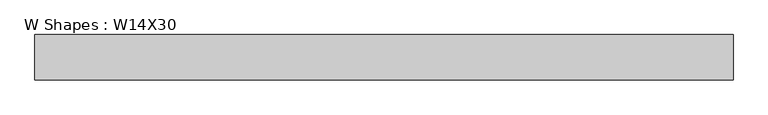
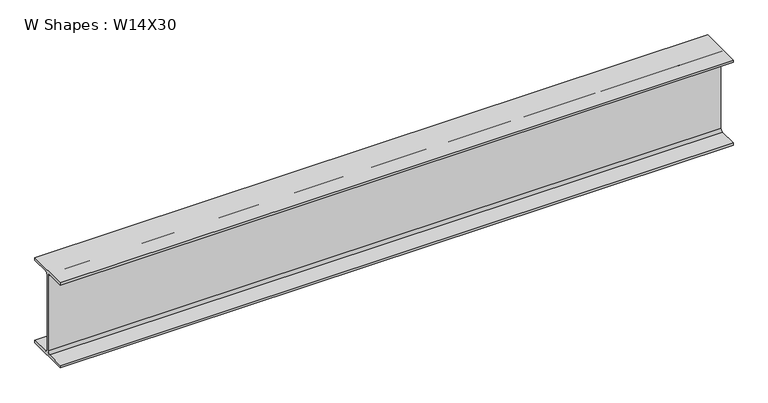
"""IFC4 building model written with IfcOpenShell, lengths in millimetres: beam geometry, W Shapes : W14X30."""

from ifc_helpers import new_model, si_unit, point, frame, frame_2d, origin, place, context, project, spatial, polyline, circle_curve, trimmed, segment, composite_curve, outline, extrude, source, transform, mapped, element, save


def w_shapes_w14x30_e8a2e8cf(model_context):
    return source(origin(), model_context, "Body", "SweptSolid", [
        extrude(outline(composite_curve([segment(polyline([(85.471, -165.481), (85.471, -175.26), (-85.471, -175.26), (-85.471, -165.481), (-13.589, -165.481)]), True, "CONTINUOUS"), segment(trimmed(circle_curve(frame_2d((-13.589, -155.321)), 10.16), [point((-13.589, -165.481))], [point((-3.429, -155.321))], True, "CARTESIAN"), True, "CONTINUOUS"), segment(polyline([(-3.429, -155.321), (-3.429, 155.321)]), True, "CONTINUOUS"), segment(trimmed(circle_curve(frame_2d((-13.589, 155.321)), 10.16), [point((-3.429, 155.321))], [point((-13.589, 165.481))], True, "CARTESIAN"), True, "CONTINUOUS"), segment(polyline([(-13.589, 165.481), (-85.471, 165.481), (-85.471, 175.26), (85.471, 175.26), (85.471, 165.481), (13.589, 165.481)]), True, "CONTINUOUS"), segment(trimmed(circle_curve(frame_2d((13.589, 155.321)), 10.16), [point((13.589, 165.481))], [point((3.429, 155.321))], True, "CARTESIAN"), True, "CONTINUOUS"), segment(polyline([(3.429, 155.321), (3.429, -155.321)]), True, "CONTINUOUS"), segment(trimmed(circle_curve(frame_2d((13.589, -155.321)), 10.16), [point((3.429, -155.321))], [point((13.589, -165.481))], True, "CARTESIAN"), True, "CONTINUOUS"), segment(polyline([(13.589, -165.481), (85.471, -165.481)]), True, "CONTINUOUS")], self_intersect=False)), frame((-1336.04, 0.0, 0.0), z_axis=(1.0, 0.0, 0.0), x_axis=(0.0, 1.0, 0.0)), (0.0, 0.0, 1.0), 2624.2095299),
    ])


if __name__ == "__main__":
    model = new_model("IFC4")
    model_context = context("Model", 3, world=origin())
    ifc_project = project(units=[si_unit("LENGTHUNIT", "METRE", prefix="MILLI")], contexts=[model_context])
    site = spatial("IfcSite", under=ifc_project)
    building = spatial("IfcBuilding", under=site)
    placement = place(None, origin())
    w_shapes_w14x30_shape = w_shapes_w14x30_e8a2e8cf(model_context)
    element("IfcBeam", 1, ObjectType="W Shapes : W14X30", at=placement, inside=building, context=model_context, shape_type="MappedRepresentation", body=[
        mapped(w_shapes_w14x30_shape, transform((0.0, 0.0, 0.0), x_axis=(1.0, 0.0, 0.0), y_axis=(0.0, 1.0, 0.0), z_axis=(0.0, 0.0, 1.0))),
    ])
    save(model, "model.ifc")

# Revit data of these elements
# Type "W Shapes : W14X30"
#   Section Name Key = "W14X30"
#   Width = 6.730"
#   Web Thickness = 0.270"
#   Web Fillet = 0.400"
#   Warping Constant = 887.00 in⁶
#   Torsional Moment of Inertia = 0.38 in⁴
#   Section Area = 8.85 in²
#   Plastic Modulus weak axis = 8.99 in³
#   Plastic Modulus strong axis = 47.30 in³
#   Perimeter = 4.441 ft²/ft
#   Nominal Weight = 30.00 lbf/ft
#   Moment of Inertia weak axis = 19.60 in⁴
#   Moment of Inertia strong axis = 291.00 in⁴
#   Height = 13.800"
#   Flange Thickness = 0.385"
#   Elastic Modulus weak axis = 5.82 in³
#   Elastic Modulus strong axis = 42.00 in³
#   Clear Web Height = 0' - 11 5/8"
#   Centroid Vertical = 6.900"
#   Centroid Horizontal = 3.365"
#   Bolt Spacing = 0' - 3 1/2"
#   Length [instance default] = 1524 mm
#   Structural Material [instance default] = Steel ASTM A992
#   Principal Axes Angle = 0
# Element 1 (IfcBeam, "W Shapes : W14X30")
#   Length = 3048 mm
#   Materials on its faces: "Steel ASTM A992"
# Materials
#   "Steel ASTM A992": class "Metal", colour RGB 199 199 199, transparency 0, Description = "Structural steel 50ksi", Cost = 0
